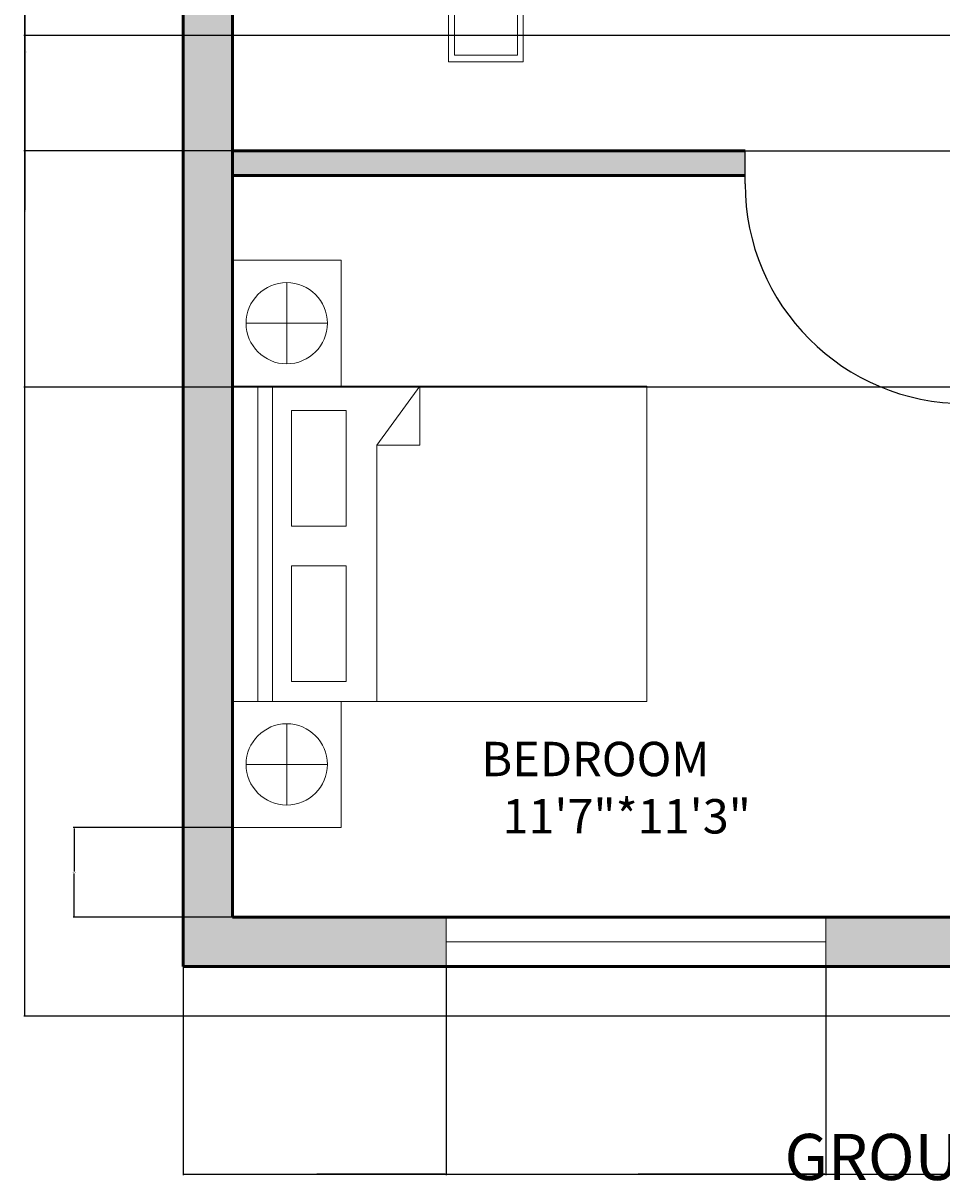
# Model space of a CAD drawing. Units: inches. Extents: x 2405 to 2823, y 1214 to 1813.
# Tile 1 of 4: x 2405 to 2572, y 1214 to 1425. Entities that reach past the tile are written whole.
import ezdxf

# ---------------------------------------------------------------- set-up
doc = ezdxf.new("R2010")
doc.units = ezdxf.units.IN
for name, color, linetype, lineweight in [('A-ANNO-DIMS', 2, 'Continuous', 18), ('A-AREA-IDEN', 30, 'Continuous', 25), ('A-WALL-PATT', 252, 'Continuous', 13), ('DOOR', 133, 'Continuous', 25), ('FUR', 10, 'Continuous', 18), ('TEXT', 30, 'Continuous', 25), ('WALL', 140, 'Continuous', 50), ('WIND', 200, 'Continuous', 18)]:
    doc.layers.add(name, color=color, linetype=linetype, lineweight=lineweight)
doc.styles.get("Standard").update_dxf_attribs({"font": 'arial.ttf'})
doc.dimstyles.get("Standard").update_dxf_attribs({"dimtxt": 0.18, "dimasz": 0.18, "dimexe": 0.18, "dimexo": 0.0625, "dimgap": 0.09, "dimtad": 0, "dimtih": 1, "dimtoh": 1, "dimdec": 4, "dimzin": 0, "dimdsep": 46, "dimtxsty": 'Standard', "dimcen": 0.09, "dimadec": 0, "dimazin": 0, "dimtfac": 1, "dimtdec": 4, "dimtofl": 0, "dimtmove": 0, "dimatfit": 3, "dimfxl": 1, "dimtolj": 1, "dimtzin": 0, "dimarcsym": 0})

# ---------------------------------------------------------------- blocks, each defined once
blk = doc.blocks.new('*U2')
for p, q in [((0, 0), (0, -6)), ((40, 0), (40, -6))]:
    blk.add_line(p, q)
blk.add_lwpolyline([(0, 0), (0, 40), (1.75, 40), (1.75, 0)], close=True)
blk.add_arc((0, 0), 40, 0, 90)
blk = doc.blocks.new('BED-DOUBLE-WITH-NIGHTSTANDS')
for p, q in [((11.49, 58.17), (11.49, 72.97)), ((91.81, 58.17), (91.81, 72.97)), ((4.09, 65.57), (18.88, 65.57)), ((84.41, 65.57), (99.2, 65.57)), ((22.97, 49.14), (69.63, 49.14)), ((69.63, 49.14), (69.63, 41.32)), ((80.32, 41.32), (69.63, 49.14)), ((69.63, 41.32), (80.32, 41.32))]:
    blk.add_line(p, q)
for points in [[(0, 75.45), (22.97, 75.45), (22.97, 55.69), (0, 55.69)], [(22.97, 75.45), (80.32, 75.45), (80.32, 0), (22.97, 0)], [(80.32, 75.45), (103.29, 75.45), (103.29, 55.69), (80.32, 55.69)], [(22.97, 70.85), (80.32, 70.85), (80.32, 68.18), (22.97, 68.18)], [(26.59, 64.68), (47.64, 64.68), (47.64, 54.75), (26.59, 54.75)], [(54.85, 64.68), (75.89, 64.68), (75.89, 54.75), (54.85, 54.75)]]:
    blk.add_lwpolyline(points, close=True)
for centre in [(11.49, 65.57), (91.81, 65.57)]:
    blk.add_circle(centre, 7.4)
blk = doc.blocks.new('CHAIR-DINING')
for p, q in [((0, 0), (0, 9.36)), ((0, 9.36), (13.56, 9.36)), ((13.56, 9.36), (13.56, 0))]:
    blk.add_line(p, q)
blk.add_lwpolyline([(1.08, 0), (12.53, 0), (12.53, 8.17), (1.08, 8.17)], close=True)
blk = doc.blocks.new('*D22')
at = {"layer": 'A-ANNO-DIMS', "color": 0, "lineweight": -2, "transparency": 16777216}
for p, q in [((2433.77, 1252.87), (2433.77, 1214.95)), ((2793.77, 1243.87), (2793.77, 1214.95)), ((2433.95, 1215.13), (2613.48, 1215.13)), ((2793.59, 1215.13), (2614.06, 1215.13))]:
    blk.add_line(p, q, dxfattribs=at)
at = {"layer": 'A-ANNO-DIMS', "color": 0, "lineweight": 100, "transparency": 16777216}
for points in [[(2433.95, 1215.16), (2433.95, 1215.1), (2433.77, 1215.13)], [(2793.59, 1215.16), (2793.59, 1215.1), (2793.77, 1215.13)]]:
    blk.add_solid(points, dxfattribs=at)
at = {"layer": 'Defpoints', "color": 0, "lineweight": 100, "transparency": 16777216}
for p in [(2433.77, 1252.93), (2793.77, 1243.93), (2793.77, 1215.13)]:
    blk.add_point(p, dxfattribs=at)
at = {"layer": 'A-ANNO-DIMS', "color": 0, "transparency": 16777216, "insert": (2613.77, 1215.13), "char_height": 0.18, "attachment_point": 5}
blk.add_mtext('\\A1;360', dxfattribs=at)
blk = doc.blocks.new('*D23')
at = {"layer": 'A-ANNO-DIMS', "color": 0, "lineweight": -2, "transparency": 16777216}
for p, q in [((2433.71, 1732.93), (2404.79, 1732.93)), ((2404.97, 1732.75), (2404.97, 1488.61)), ((2404.97, 1244.11), (2404.97, 1488.25)), ((2586.21, 1243.93), (2404.79, 1243.93))]:
    blk.add_line(p, q, dxfattribs=at)
at = {"layer": 'A-ANNO-DIMS', "color": 0, "lineweight": 100, "transparency": 16777216}
for points in [[(2404.94, 1732.75), (2405, 1732.75), (2404.97, 1732.93)], [(2404.94, 1244.11), (2405, 1244.11), (2404.97, 1243.93)]]:
    blk.add_solid(points, dxfattribs=at)
at = {"layer": 'Defpoints', "color": 0, "lineweight": 100, "transparency": 16777216}
for p in [(2433.77, 1732.93), (2404.97, 1243.93), (2586.27, 1243.93)]:
    blk.add_point(p, dxfattribs=at)
at = {"layer": 'A-ANNO-DIMS', "color": 0, "transparency": 16777216, "insert": (2404.97, 1488.43), "char_height": 0.18, "attachment_point": 5}
blk.add_mtext('\\A1;489', dxfattribs=at)
blk = doc.blocks.new('*D25')
at = {"layer": 'A-ANNO-DIMS', "color": 0, "lineweight": -2, "transparency": 16777216}
for p, q in [((2442.71, 1437.52), (2404.79, 1437.52)), ((2404.97, 1437.34), (2404.97, 1419.66)), ((2404.97, 1401.61), (2404.97, 1419.29)), ((2442.71, 1401.43), (2404.79, 1401.43))]:
    blk.add_line(p, q, dxfattribs=at)
at = {"layer": 'A-ANNO-DIMS', "color": 0, "lineweight": 100, "transparency": 16777216}
for points in [[(2404.94, 1437.34), (2405, 1437.34), (2404.97, 1437.52)], [(2404.94, 1401.61), (2405, 1401.61), (2404.97, 1401.43)]]:
    blk.add_solid(points, dxfattribs=at)
at = {"layer": 'Defpoints', "color": 0, "lineweight": 100, "transparency": 16777216}
for p in [(2442.77, 1437.52), (2404.97, 1401.43), (2442.77, 1401.43)]:
    blk.add_point(p, dxfattribs=at)
at = {"layer": 'A-ANNO-DIMS', "color": 0, "transparency": 16777216, "insert": (2404.97, 1419.47), "char_height": 0.18, "attachment_point": 5}
blk.add_mtext('\\A1;36.09', dxfattribs=at)
blk = doc.blocks.new('*D30')
at = {"layer": 'A-ANNO-DIMS', "color": 0, "lineweight": -2, "transparency": 16777216}
for p, q in [((2433.77, 1252.87), (2433.77, 1214.95)), ((2481.68, 1252.87), (2481.68, 1214.95)), ((2433.95, 1215.13), (2457.34, 1215.13)), ((2481.5, 1215.13), (2458.1, 1215.13))]:
    blk.add_line(p, q, dxfattribs=at)
at = {"layer": 'A-ANNO-DIMS', "color": 0, "lineweight": 100, "transparency": 16777216}
for points in [[(2433.95, 1215.16), (2433.95, 1215.1), (2433.77, 1215.13)], [(2481.5, 1215.16), (2481.5, 1215.1), (2481.68, 1215.13)]]:
    blk.add_solid(points, dxfattribs=at)
at = {"layer": 'Defpoints', "color": 0, "lineweight": 100, "transparency": 16777216}
for p in [(2433.77, 1252.93), (2481.68, 1252.93), (2481.68, 1215.13)]:
    blk.add_point(p, dxfattribs=at)
at = {"layer": 'A-ANNO-DIMS', "color": 0, "transparency": 16777216, "insert": (2457.72, 1215.13), "char_height": 0.18, "attachment_point": 5}
blk.add_mtext('\\A1;47.91', dxfattribs=at)
blk = doc.blocks.new('*D31')
at = {"layer": 'A-ANNO-DIMS', "color": 0, "lineweight": -2, "transparency": 16777216}
for p, q in [((2481.68, 1252.87), (2481.68, 1214.95)), ((2550.8, 1252.87), (2550.8, 1214.95)), ((2481.86, 1215.13), (2515.85, 1215.13)), ((2550.62, 1215.13), (2516.63, 1215.13))]:
    blk.add_line(p, q, dxfattribs=at)
at = {"layer": 'A-ANNO-DIMS', "color": 0, "lineweight": 100, "transparency": 16777216}
for points in [[(2481.86, 1215.16), (2481.86, 1215.1), (2481.68, 1215.13)], [(2550.62, 1215.16), (2550.62, 1215.1), (2550.8, 1215.13)]]:
    blk.add_solid(points, dxfattribs=at)
at = {"layer": 'Defpoints', "color": 0, "lineweight": 100, "transparency": 16777216}
for p in [(2481.68, 1252.93), (2550.8, 1252.93), (2550.8, 1215.13)]:
    blk.add_point(p, dxfattribs=at)
at = {"layer": 'A-ANNO-DIMS', "color": 0, "transparency": 16777216, "insert": (2516.24, 1215.13), "char_height": 0.18, "attachment_point": 5}
blk.add_mtext('\\A1;69.12', dxfattribs=at)
blk = doc.blocks.new('*D34')
at = {"layer": 'A-ANNO-DIMS', "color": 0, "lineweight": -2, "transparency": 16777216}
for p, q in [((2652.71, 1422.43), (2404.79, 1422.43)), ((2404.97, 1422.25), (2404.97, 1390.61)), ((2404.97, 1358.61), (2404.97, 1390.25)), ((2652.71, 1358.43), (2404.79, 1358.43))]:
    blk.add_line(p, q, dxfattribs=at)
at = {"layer": 'A-ANNO-DIMS', "color": 0, "lineweight": 100, "transparency": 16777216}
for points in [[(2404.94, 1422.25), (2405, 1422.25), (2404.97, 1422.43)], [(2404.94, 1358.61), (2405, 1358.61), (2404.97, 1358.43)]]:
    blk.add_solid(points, dxfattribs=at)
at = {"layer": 'Defpoints', "color": 0, "lineweight": 100, "transparency": 16777216}
for p in [(2404.97, 1422.43), (2652.77, 1422.43), (2652.77, 1358.43)]:
    blk.add_point(p, dxfattribs=at)
at = {"layer": 'A-ANNO-DIMS', "color": 0, "transparency": 16777216, "insert": (2404.97, 1390.43), "char_height": 0.18, "attachment_point": 5}
blk.add_mtext('\\A1;64', dxfattribs=at)
blk = doc.blocks.new('*D49')
at = {"layer": 'A-ANNO-DIMS', "color": 0, "lineweight": -2, "transparency": 16777216}
for p, q in [((2442.77, 1401.49), (2442.77, 1812.91)), ((2442.95, 1812.73), (2459.64, 1812.73)), ((2477.12, 1812.73), (2460.43, 1812.73)), ((2477.3, 1427.08), (2477.3, 1812.91))]:
    blk.add_line(p, q, dxfattribs=at)
at = {"layer": 'A-ANNO-DIMS', "color": 0, "lineweight": 100, "transparency": 16777216}
for points in [[(2442.95, 1812.76), (2442.95, 1812.7), (2442.77, 1812.73)], [(2477.12, 1812.76), (2477.12, 1812.7), (2477.3, 1812.73)]]:
    blk.add_solid(points, dxfattribs=at)
at = {"layer": 'Defpoints', "color": 0, "lineweight": 100, "transparency": 16777216}
for p in [(2477.3, 1812.73), (2477.3, 1427.01), (2442.77, 1401.43)]:
    blk.add_point(p, dxfattribs=at)
at = {"layer": 'A-ANNO-DIMS', "color": 0, "transparency": 16777216, "insert": (2460.03, 1812.73), "char_height": 0.18, "attachment_point": 5}
blk.add_mtext('\\A1;34.53', dxfattribs=at)
blk = doc.blocks.new('*D50')
at = {"layer": 'A-ANNO-DIMS', "color": 0, "lineweight": -2, "transparency": 16777216}
for p, q in [((2477.36, 1427.01), (2822.75, 1427.01)), ((2822.57, 1426.83), (2822.57, 1414.4)), ((2822.57, 1401.61), (2822.57, 1414.04)), ((2442.83, 1401.43), (2822.75, 1401.43))]:
    blk.add_line(p, q, dxfattribs=at)
at = {"layer": 'A-ANNO-DIMS', "color": 0, "lineweight": 100, "transparency": 16777216}
for points in [[(2822.54, 1426.83), (2822.6, 1426.83), (2822.57, 1427.01)], [(2822.54, 1401.61), (2822.6, 1401.61), (2822.57, 1401.43)]]:
    blk.add_solid(points, dxfattribs=at)
at = {"layer": 'Defpoints', "color": 0, "lineweight": 100, "transparency": 16777216}
for p in [(2477.3, 1427.01), (2822.57, 1427.01), (2442.77, 1401.43)]:
    blk.add_point(p, dxfattribs=at)
at = {"layer": 'A-ANNO-DIMS', "color": 0, "transparency": 16777216, "insert": (2822.57, 1414.22), "char_height": 0.18, "attachment_point": 5}
blk.add_mtext('\\A1;25.584', dxfattribs=at)
blk = doc.blocks.new('*D54')
at = {"layer": 'A-ANNO-DIMS', "color": 0, "lineweight": -2, "transparency": 16777216}
for p, q in [((2442.71, 1278.25), (2413.79, 1278.25)), ((2413.97, 1278.07), (2413.97, 1270.27)), ((2413.97, 1262.11), (2413.97, 1269.91)), ((2442.71, 1261.93), (2413.79, 1261.93))]:
    blk.add_line(p, q, dxfattribs=at)
at = {"layer": 'A-ANNO-DIMS', "color": 0, "lineweight": 100, "transparency": 16777216}
for points in [[(2413.94, 1278.07), (2414, 1278.07), (2413.97, 1278.25)], [(2413.94, 1262.11), (2414, 1262.11), (2413.97, 1261.93)]]:
    blk.add_solid(points, dxfattribs=at)
at = {"layer": 'Defpoints', "color": 0, "lineweight": 100, "transparency": 16777216}
for p in [(2413.97, 1278.25), (2442.77, 1278.25), (2442.77, 1261.93)]:
    blk.add_point(p, dxfattribs=at)
at = {"layer": 'A-ANNO-DIMS', "color": 0, "transparency": 16777216, "insert": (2413.97, 1270.09), "char_height": 0.18, "attachment_point": 5}
blk.add_mtext('\\A1;16.32', dxfattribs=at)

msp = doc.modelspace()

# ---------------------------------------------------------------- hatches: boundary and pattern name
at = {"layer": 'A-WALL-PATT'}
h = msp.add_hatch(color=256, dxfattribs=at)
h.dxf.hatch_style = 1
h.paths.add_polyline_path([(2601.7679, 1732.9303), (2433.7679, 1732.9303), (2433.7679, 1680.7368), (2442.7679, 1680.7368), (2442.7679, 1723.9303), (2574.7679, 1723.9303), (2601.7679, 1723.9303)])
h.paths.add_polyline_path([(2793.7679, 1732.9303), (2622.7552, 1732.9303), (2622.7552, 1723.9303), (2622.7679, 1723.9303), (2645.2679, 1723.9303), (2784.7679, 1723.9303), (2784.7679, 1680.7368), (2793.7679, 1680.7368)])
h.paths.add_polyline_path([(2442.7679, 1605.111), (2433.7679, 1605.111), (2433.7679, 1513.1454), (2442.7679, 1513.1454), (2442.7679, 1563.4303)])
h.paths.add_polyline_path([(2531.8067, 1567.9303), (2442.7679, 1567.9303), (2442.7679, 1563.4303), (2531.8067, 1563.4303)])
h.paths.add_polyline_path([(2793.7679, 1605.111), (2784.7679, 1605.111), (2784.7679, 1555.6662), (2793.7679, 1555.6662)])
h.paths.add_polyline_path([(2784.7679, 1567.9303), (2691.5187, 1567.9303), (2691.5187, 1563.4303), (2784.7679, 1563.4303)])
h.paths.add_polyline_path([(2649.7679, 1611.4303), (2645.2679, 1611.4303), (2645.2679, 1563.4303), (2651.5187, 1563.4303), (2651.5187, 1567.9303), (2649.7679, 1567.9303)])
h.paths.add_polyline_path([(2581.5295, 1614.9584), (2581.5295, 1615.9303), (2579.2679, 1615.9303), (2579.2679, 1611.4303), (2581.5295, 1611.4303)])
h.paths.add_polyline_path([(2579.2679, 1723.9303), (2574.7679, 1723.9303), (2574.7679, 1567.9303), (2571.8067, 1567.9303), (2571.8067, 1563.4303), (2579.2679, 1563.4303)])
h.paths.add_polyline_path([(2649.7679, 1723.9303), (2645.2679, 1723.9303), (2645.2679, 1615.9303), (2605.0298, 1615.9303, -0.01033406), (2605.0499, 1614.9584), (2605.0499, 1611.4303), (2649.7679, 1611.4303)])
h.paths.add_polyline_path([(2793.7679, 1523.737), (2784.7679, 1523.737), (2784.7679, 1492.9303), (2793.7679, 1492.9303)])
h.paths.add_polyline_path([(2793.7679, 1446.4039), (2784.7679, 1446.4039), (2784.7679, 1426.9303), (2784.7679, 1412.6503), (2793.7679, 1412.6503)])
h.paths.add_polyline_path([(2652.7679, 1467.3906), (2648.2679, 1467.3906), (2648.2679, 1422.4303), (2784.7679, 1422.4303), (2784.7679, 1426.9303), (2652.7679, 1426.9303)])
h.paths.add_polyline_path([(2696.2679, 1515.4303), (2648.2679, 1515.4303), (2648.2679, 1507.3906), (2652.7679, 1507.3906), (2652.7679, 1510.9303), (2696.2679, 1510.9303)])
h.paths.add_polyline_path([(2784.7679, 1515.4303), (2700.7679, 1515.4303), (2696.2679, 1515.4303), (2696.2679, 1510.9303), (2784.7679, 1510.9303)])
h.paths.add_polyline_path([(2700.7679, 1522.7934), (2696.2679, 1522.7934), (2696.2679, 1515.4303), (2700.7679, 1515.4303)])
h.paths.add_polyline_path([(2700.7679, 1563.4303), (2696.2679, 1563.4303), (2696.2679, 1557.1044), (2700.7679, 1557.1044)])
h.paths.add_polyline_path([(2442.7679, 1437.5196), (2433.7679, 1437.5196), (2433.7679, 1252.9303), (2481.6786, 1252.9303), (2481.6786, 1261.9303), (2442.7679, 1261.9303)])
h.paths.add_polyline_path([(2536.0913, 1401.4303), (2442.7679, 1401.4303), (2442.7679, 1396.9303), (2536.0913, 1396.9303)])
h.paths.add_polyline_path([(2784.7679, 1358.4303), (2630.4061, 1358.4303), (2630.4061, 1353.9303), (2784.7679, 1353.9303)])
h.paths.add_polyline_path([(2793.7679, 1366.1239), (2784.7679, 1366.1239), (2784.7679, 1261.9303), (2784.7679, 1243.9303), (2793.7679, 1243.9303), (2793.7679, 1260.2097)])
h.paths.add_polyline_path([(2590.4061, 1358.4303), (2586.2679, 1358.4303), (2586.2679, 1353.9303), (2590.4061, 1353.9303)])
h.paths.add_polyline_path([(2586.2679, 1353.9303), (2586.2679, 1401.4303), (2576.0913, 1401.4303), (2576.0913, 1396.9303), (2581.7679, 1396.9303), (2581.7679, 1261.9303), (2586.2679, 1261.9303)])
h.paths.add_polyline_path([(2586.2679, 1261.9303), (2581.7679, 1261.9303), (2550.8023, 1261.9303), (2550.8023, 1252.9303), (2586.2679, 1252.9303)])

# ---------------------------------------------------------------- linework, layer by layer
at = {"layer": 'WALL'}
for p, q in [((2433.7679, 1252.9303), (2433.7679, 1732.9303)), ((2442.7679, 1261.9303), (2442.7679, 1723.9303)), ((2442.7679, 1563.4303), (2442.7679, 1401.4303)), ((2442.7679, 1401.4303), (2536.0913, 1401.4303)), ((2442.7679, 1396.9303), (2536.0913, 1396.9303)), ((2784.7679, 1261.9303), (2442.7679, 1261.9303)), ((2784.7679, 1252.9303), (2433.7679, 1252.9303))]:
    msp.add_line(p, q, dxfattribs=at)
at = {"layer": 'WIND'}
msp.add_line((2481.6786, 1257.4303), (2550.8023, 1257.4303), dxfattribs=at)
msp.add_lwpolyline([(2481.6786, 1261.9303), (2550.8023, 1261.9303), (2550.8023, 1252.9303), (2481.6786, 1252.9303)], close=True, dxfattribs=at)

# ---------------------------------------------------------------- block references
at = {"layer": 'DOOR', "rotation": 180}
msp.add_blockref('*U2', (2576.0913, 1395.4303), dxfattribs=at)
at = {"layer": 'FUR', "extrusion": (0, 0, -1), "zscale": -1, "rotation": 180}
msp.add_blockref('CHAIR-DINING', (-2482.119, 1427.0142), dxfattribs=at)
at = {"layer": 'FUR', "rotation": 90.00000000000017}
msp.add_blockref('BED-DOUBLE-WITH-NIGHTSTANDS', (2518.2162, 1278.2493), dxfattribs=at)

# ---------------------------------------------------------------- texts
at = {"layer": 'A-AREA-IDEN', "insert": (2488.084, 1293.851), "char_height": 6.256044, "attachment_point": 1}
msp.add_mtext_dynamic_manual_height_columns('BEDROOM\\P  11\'7"*11\'3"', width=135.493128, gutter_width=31.2802, heights=[0], dxfattribs=at)
at = {"layer": 'TEXT', "insert": (2543.2701, 1222.4779), "char_height": 8.397982, "attachment_point": 1}
msp.add_mtext_dynamic_manual_height_columns('GROUND FLOOR PLAN', width=725.174894, gutter_width=41.9899, heights=[0], dxfattribs=at)

# ---------------------------------------------------------------- dimensions: what is measured, and where the dimension line sits
at = {"layer": 'A-ANNO-DIMS'}
for base, p1, p2, override, picture, middle in [((2477.2955, 1812.7303), (2442.7679, 1401.4303), (2477.2955, 1427.0139), {"dimdec": 2, "dimlfac": 1, "dimrnd": 0, "dimzin": 0, "dimdsep": 46, "dimlunit": 2}, '*D49', (2460.0317, 1812.7303)), ((2793.7679, 1215.1303), (2433.7679, 1252.9303), (2793.7679, 1243.9303), {"dimdec": 0, "dimlfac": 1, "dimrnd": 0, "dimzin": 0, "dimdsep": 46, "dimlunit": 2}, '*D22', (2613.7679, 1215.1303)), ((2481.6786, 1215.1303), (2433.7679, 1252.9303), (2481.6786, 1252.9303), {"dimdec": 2, "dimlfac": 1, "dimrnd": 0, "dimzin": 0, "dimdsep": 46, "dimlunit": 2}, '*D30', (2457.7233, 1215.1303)), ((2550.8023, 1215.1303), (2481.6786, 1252.9303), (2550.8023, 1252.9303), {"dimdec": 2, "dimlfac": 1, "dimrnd": 0, "dimzin": 0, "dimdsep": 46, "dimlunit": 2}, '*D31', (2516.2405, 1215.1303))]:
    dim = msp.add_linear_dim(base=base, p1=p1, p2=p2, dimstyle='Standard', override=override, dxfattribs=at)
    dim.commit()
    dim.dimension.update_dxf_attribs({"geometry": picture, "text_midpoint": middle})
for base, p1, p2, override, picture, middle in [((2404.9679, 1243.9303), (2433.7679, 1732.9303), (2586.2679, 1243.9303), {"dimdec": 0, "dimlfac": 1, "dimrnd": 0, "dimzin": 0, "dimdsep": 46, "dimlunit": 2}, '*D23', (2404.9679, 1488.4303)), ((2404.9679, 1401.4303), (2442.7679, 1437.5196), (2442.7679, 1401.4303), {"dimdec": 2, "dimlfac": 1, "dimrnd": 0, "dimzin": 0, "dimdsep": 46, "dimlunit": 2}, '*D25', (2404.9679, 1419.475)), ((2822.5679, 1427.0139), (2442.7679, 1401.4303), (2477.2955, 1427.0139), {"dimdec": 3, "dimlfac": 1, "dimrnd": 0, "dimzin": 0, "dimdsep": 46, "dimlunit": 2}, '*D50', (2822.5679, 1414.2221)), ((2404.9679, 1422.4303), (2652.7679, 1358.4303), (2652.7679, 1422.4303), {"dimdec": 0, "dimlfac": 1, "dimrnd": 0, "dimzin": 0, "dimdsep": 46, "dimlunit": 2}, '*D34', (2404.9679, 1390.4303)), ((2413.9679, 1278.2492), (2442.7679, 1261.9303), (2442.7679, 1278.2492), {"dimdec": 2, "dimlfac": 1, "dimrnd": 0, "dimzin": 0, "dimdsep": 46, "dimlunit": 2}, '*D54', (2413.9679, 1270.0898))]:
    dim = msp.add_linear_dim(base=base, p1=p1, p2=p2, angle=90, dimstyle='Standard', override=override, dxfattribs=at)
    dim.commit()
    dim.dimension.update_dxf_attribs({"geometry": picture, "text_midpoint": middle})

doc.saveas('drawing.dxf')
